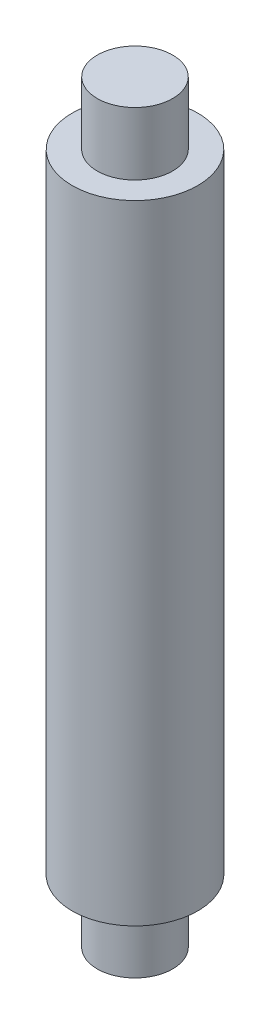
from build123d import *


with BuildPart() as part:
    # Shaft Profile Sketch → Stepped Shaft Ø20 Journals Ø12 (revolve)
    with BuildSketch(Plane.XY, mode=Mode.PRIVATE) as stepped_shaft_20_journals_12_sk:
        Polygon((0, 0), (6, 0), (6, 10), (10, 10), (10, 110), (6, 110), (6, 120), (0, 120), align=None)
    revolve(stepped_shaft_20_journals_12_sk.sketch.rotate(Axis((0, 120, 0), (0, -1, 0)), 90), axis=Axis((0, 120, 0), (0, -1, 0)))


solid = part.part
